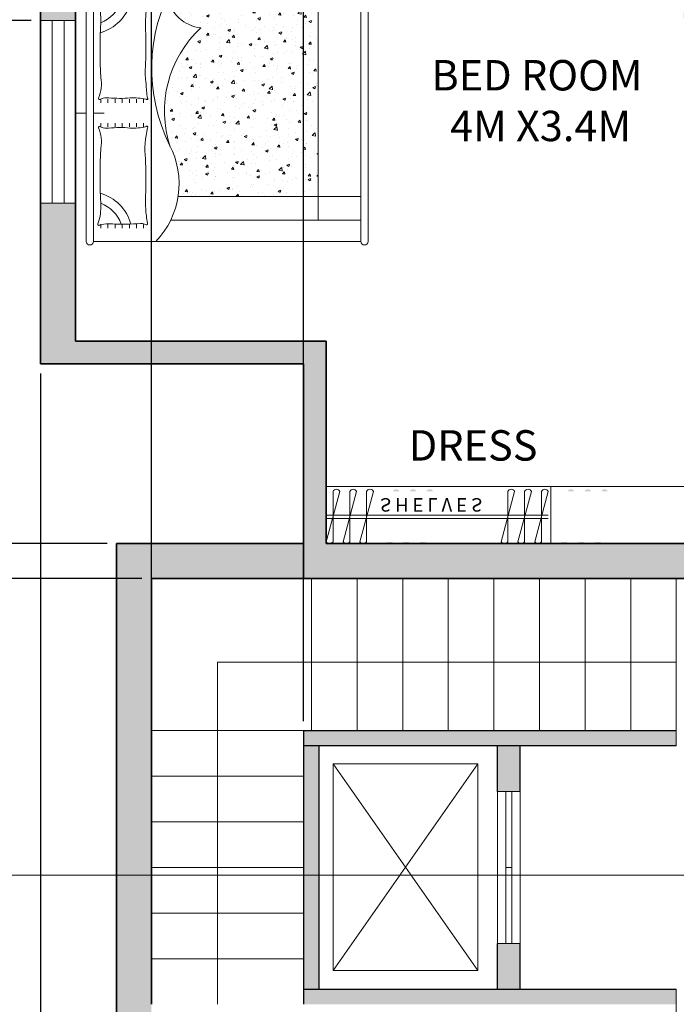
# Model space of a CAD drawing. Units: metres. Extents: x 2031 to 2061.8, y 1886.4 to 1909.8.
# Tile 5 of 10: x 2036.1 to 2040.4, y 1896.6 to 1903. Entities that reach past the tile are written whole.
import ezdxf

# ---------------------------------------------------------------- set-up
doc = ezdxf.new("R2010")
doc.units = ezdxf.units.M
for name, color, linetype, lineweight in [('A-ANNO-DIMS', 2, 'Continuous', 18), ('A-ANNO-SYMB', 7, 'Continuous', 18), ('A-AREA-IDEN', 7, 'Continuous', 18), ('A-FLOR-CASE', 8, 'Continuous', 18), ('A-FLOR-EVTR', 4, 'Continuous', 18), ('A-FLOR-STRS', 7, 'Continuous', 18), ('A-FLOR-STRS-PATH', 1, 'Continuous', 13), ('A-WALL-PATT', 252, 'Continuous', 13), ('furniture', 24, 'Continuous', 13), ('inner walls', 4, 'Continuous', 25), ('windows', 30, 'Continuous', 18)]:
    doc.layers.add(name, color=color, linetype=linetype, lineweight=lineweight)
doc.layers.add('outer walls', color=1, linetype='Continuous', lineweight=35, plot=False)
doc.styles.get("Standard").update_dxf_attribs({"font": 'arial.ttf'})
doc.dimstyles.get("Standard").update_dxf_attribs({"dimtxt": 0.18, "dimasz": 0.18, "dimexe": 0.18, "dimexo": 0.0625, "dimgap": 0.09, "dimtad": 0, "dimtih": 1, "dimtoh": 1, "dimdec": 4, "dimzin": 0, "dimdsep": 46, "dimtxsty": 'Standard', "dimcen": 0.09, "dimadec": 0, "dimazin": 0, "dimtfac": 1, "dimtdec": 4, "dimtofl": 0, "dimtmove": 0, "dimatfit": 3, "dimfxl": 1, "dimtolj": 1, "dimtzin": 0, "dimarcsym": 0})

# ---------------------------------------------------------------- blocks, each defined once
blk = doc.blocks.new('bed')
at = {"layer": 'furniture'}
h = blk.add_hatch(dxfattribs=at)
h.set_pattern_fill('AR-CONC', color=256, angle=-90.00000000000003, style=0)
h.set_pattern_definition([(320, (0, 2.380000000001032), (-0.6275213498259539, -7.172601826007534), [0.75, -8.25]), (265, (0, 2.380000000001032), (7.521921337000119, 1.387513336129997), [0.6, -6.599999999999999]), (10.45139999999999, (-0.0522933999999964, 1.782283200001032), (6.894395420609534, -5.785093817140218), [0.6374019000000001, -7.011421119999999]), (316.1842, (2, 2.380000000001032), (-1.655190143290184, -10.67241048625644), [1.125, -12.375]), (6.635599999999979, (1.862066929999997, 1.490632550001038), (9.741178709004412, -9.346627055487035), [0.956102879999999, -10.51712999999998]), (261.1842, (2, 2.380000000001032), (9.741186009253243, -9.346619451336275), [0.8999999999999989, -9.899999999999984]), (291, (1.5, 1.380000000001032), (-4.02618890665339, -5.969070521184614), [0.75, -8.25]), (236, (1.5, 1.380000000001032), (7.251500450468529, -2.433153319215819), [0.6, -6.599999999999999]), (341.4514, (1.164483939999996, 0.8825776700010266), (3.22530496709952, -8.402226285814901), [0.6374019000000001, -7.011421119999999]), (307.4999999999999, (0, 2.380000000001032), (3.328938538313114, -0.121598553172908), [0, -6.519999999999999, 0, -6.7, 0, -6.625]), (277.5, (0, 2.380000000001032), (3.944117118823601, -2.630695374421487), [0, -3.819999999999999, 0, -6.37, 0, -2.524999999999999]), (237.5, (0, 4.610000000001036), (-0.2255487173438, -5.33822436172409), [0, -2.5, 0, -7.799999999999999, 0, -10.35]), (227.5, (0, 5.610000000001036), (1.001049823323174, -5.831861693423862), [0, -3.25, 0, -5.179999999999999, 0, -7.349999999999999])])
h.paths.add_polyline_path([(30.01221964123038, -67.99999999999999), (30.01221964123036, -26.4972098666525, 0.2630430180581192), (23.90476957024844, -35.1500155485824, 0.2934236934375176), (-9.177957282599145, -26.46678060096597, -0.1566832162072435), (-23.39221964123496, -28.71851562074189), (-23.39221964123494, -67.99999999999999)])
for p, q in [((0, -3), (0, 0)), ((36.01221964123033, -3), (-36.01221964123033, -3)), ((-36.01221964123033, -5.000000000000028), (-36.01221964123027, -80)), ((36.01221964123033, -5.000000000000042), (-36.01221964123033, -5.000000000000028)), ((0, -8.000000000000043), (0, -5.000000000000042)), ((36.01221964123039, -79.99999999999999), (36.01221964123033, -5.000000000000042)), ((-31.23716250644156, -7.067621994530554), (-32.23716250644157, -7.067621994530554)), ((-3.810600647213163, -7.067621994530554), (-2.810600647213163, -7.067621994530554)), ((3.894900133777696, -7.067621994530526), (2.894900133777696, -7.067621994530526)), ((31.62837541028949, -7.067621994530526), (32.62837541028949, -7.067621994530526)), ((-31.23716250644156, -9.067621994530555), (-32.23716250644157, -9.067621994530555)), ((-3.810600647213163, -9.067621994530555), (-2.810600647213163, -9.067621994530555)), ((3.894900133777696, -9.067621994530526), (2.894900133777696, -9.067621994530526)), ((31.62837541028949, -9.067621994530526), (32.62837541028949, -9.067621994530526)), ((-31.23716250644156, -11.06762199453055), (-32.23716250644157, -11.06762199453055)), ((-31.23716250644156, -13.06762199453055), (-32.23716250644157, -13.06762199453055)), ((-3.810600647213163, -11.06762199453055), (-2.810600647213163, -11.06762199453055)), ((-3.810600647213163, -13.06762199453055), (-2.810600647213163, -13.06762199453055)), ((3.894900133777696, -11.06762199453052), (2.894900133777696, -11.06762199453052)), ((3.894900133777696, -13.06762199453052), (2.894900133777696, -13.06762199453052)), ((31.62837541028949, -11.06762199453052), (32.62837541028949, -11.06762199453052)), ((31.62837541028949, -13.06762199453052), (32.62837541028949, -13.06762199453052)), ((-31.23716250644156, -15.06762199453055), (-32.23716250644157, -15.06762199453055)), ((-3.810600647213163, -15.06762199453055), (-2.810600647213163, -15.06762199453055)), ((3.894900133777696, -15.06762199453052), (2.894900133777696, -15.06762199453052)), ((31.62837541028949, -15.06762199453052), (32.62837541028949, -15.06762199453052)), ((-31.23716250644156, -17.06762199453055), (-32.23716250644157, -17.06762199453055)), ((-31.23716250644156, -19.06762199453055), (-32.23716250644157, -19.06762199453055)), ((-3.810600647213163, -17.06762199453055), (-2.810600647213163, -17.06762199453055)), ((-3.810600647213163, -19.06762199453055), (-2.810600647213163, -19.06762199453055)), ((3.894900133777696, -17.06762199453052), (2.894900133777696, -17.06762199453052)), ((3.894900133777696, -19.06762199453052), (2.894900133777696, -19.06762199453052)), ((31.62837541028949, -17.06762199453052), (32.62837541028949, -17.06762199453052)), ((31.62837541028949, -19.06762199453052), (32.62837541028949, -19.06762199453052)), ((-36.01221964123027, -80), (36.01221964123039, -79.99999999999997)), ((-36.01221964123027, -82), (36.01221964123039, -82))]:
    blk.add_line(p, q, dxfattribs=at)
at = {"layer": 'furniture', "ltscale": 5}
blk.add_line((-30.0122196412303, -26.65900214866815), (-30.01221964123028, -80), dxfattribs=at)
at = {"layer": 'furniture', "ltscale": 7}
blk.add_line((30.01221964123039, -79.99999999999999), (30.01221964123036, -26.4972098666525), dxfattribs=at)
at = {"layer": 'furniture', "ltscale": 0.3}
for p, q in [((-23.39221964123493, -80.00000000000003), (-23.39221964123496, -28.71851562074188)), ((-30.01221964123028, -67.99999999999999), (30.01221964123039, -67.99999999999999))]:
    blk.add_line(p, q, dxfattribs=at)
at = {"layer": 'furniture'}
for centre, radius, start, end in [((-35.95310404783035, -4.000000000000014), 1.001745802777857, 93.38313670775338, 266.6168632922466), ((35.95310404783047, -4.000000000000014), 1.001745802777857, 273.3831367077534, 86.61686329224663), ((-31.09685452420217, -6.56812628935117), 0.3815901177143176, 35.89755946985184, 208.6271807330242), ((-44.4434251214767, -13.85312857714783), 14.82374463825802, 27.16285943351717, 28.62718073212637), ((-46.75951437957865, -9.65138206848897), 15.71579241958107, 357.4803608088326, 9.395608387614068), ((-34.45294545533051, -3.506108501804959), 9.853247350176973, 289.8695209624031, 338.9842964810487), ((-34.45294545533051, -3.506108501804959), 12.47479548168961, 286.0319050224358, 344.1205283884622), ((-26.34909713879518, 6.677823774407073), 13.75788850886336, 251.1782289026713, 273.3982224065857), ((-18.01528168092849, -163.5963416214672), 156.7209082093599, 87.00321809951629, 92.74968346925495), ((-8.031939823939297, 2.030581047412752), 9.294330538692307, 258.8960367609226, 294.7184225587751), ((0.254091396095987, -8.800915214962217), 4.494229367051207, 159.014640107615, 186.2730421081171), ((-4.029449448298862, -6.668977911985379), 0.2818061021667602, 335.7259061638442, 114.3030308467571), ((3.223958981487498, -9.94006998173215), 7.675076275868892, 155.7259061638442, 159.0146401085631), ((4.113748934860268, -6.668977911985379), 0.2818061021635516, 65.69696915417202, 204.2740938370052), ((-3.139659494904833, -9.940069981732137), 7.675076275868892, 20.98535989143595, 24.27409383615427), ((-0.1697919095242355, -8.800915214962217), 4.494229367051207, 353.7269578918828, 20.98535989238499), ((8.116239310533615, 2.030581047735168), 9.294330539002221, 245.2815774418415, 281.1039632384965), ((18.09958116748922, -163.5963416214399), 156.7209082093326, 87.2503165307418, 92.99678190048373), ((34.53724494190226, -3.506108501789682), 12.47479548168961, 195.8794716115377, 253.9680949775642), ((34.53724494190226, -3.506108501789682), 9.853247350176973, 201.0157035189505, 250.1304790375968), ((26.43339662535652, 6.677823774423444), 13.75788850886336, 266.6017775934111, 288.8217710973251), ((31.18115401076358, -6.568126289351184), 0.3815901177179044, 331.3728192669758, 144.1024405301472), ((46.84381386614001, -9.651382068520647), 15.71579241958353, 170.6043916115409, 182.5196391911672), ((44.52772460803806, -13.85312857714784), 14.82374463825802, 151.3728192678729, 152.8371405664821), ((54.88285648445511, -13.16191061182081), 85.98801403775587, 178.1208768196816, 183.3613129440673), ((-32.81622258778788, -12.43616332427339), 28.77528664700029, 354.3784002715227, 6.27304210895588), ((32.90052207435963, -12.43616332427341), 28.77528664700055, 173.7269578910441, 185.6215997284773), ((-54.79855699787332, -13.1619106118885), 85.98801403775471, 356.6386870559327, 1.87912318031836), ((-28.61556435462791, 31.03444768063454), 42.31456350822244, 266.4835611990511, 266.6487421238194), ((28.69986384117891, 31.03444768073385), 42.31456350831875, 273.3512578762066, 273.5164388009489), ((12.27920019974715, -16.10835590841725), 16.48064095036883, 177.0317121189266, 192.8677860199701), ((-12.19490071317551, -16.10835590841725), 16.48064095036894, 347.1322139800299, 2.968287881073314), ((-34.12771521855714, -18.41167218428833), 3.177308659740759, 342.7808628527732, 3.755021134780372), ((34.21201470513921, -18.41167218428845), 3.177308659740705, 176.2449788652196, 197.2191371472267), ((-31.05019458355673, -19.91479358257859), 0.2912925215689113, 147.6219291273817, 311.93432899363), ((-33.19532486499685, -18.55460390606353), 2.248727139855352, 327.6219291288709, 339.224552802207), ((-24.39731400277299, -58.0065508966982), 38.42172354635978, 93.51643880178425, 99.67664784205135), ((-24.51665474671893, -56.06449133928439), 36.47600066328987, 86.48356119821578, 93.51643880178425), ((-18.48842024981553, 70.49496359167773), 90.23180174042126, 267.5920770069633, 273.6328801943956), ((-10.30534078399284, -44.95285539311296), 25.51674577343078, 75.95197577712642, 95.54518109318596), ((12.50744191168894, -69.71437404891591), 48.3828132966499, 60.93454900685955, 116.3226601669859), ((-3.947726608991956, -19.99033763805275), 0.2654728058058112, 231.9004795059564, 52.89022406852256), ((4.032026095563765, -19.99033763805275), 0.2654728058058112, 127.1097759314774, 308.0995204940429), ((7.570216687580227, -34.67789736270967), 14.86666553287629, 87.39755039330738, 103.1191401867811), ((11.43897390287765, -34.80624327566366), 15.31635237680183, 84.69404282866213, 102.035481886755), ((18.57271973638731, 70.4949635916777), 90.23180174042125, 266.3671198056044, 272.4079229930367), ((24.6009542333012, -56.0644913392844), 36.47600066328987, 86.48356119821578, 93.51643880178425), ((24.48161348934542, -58.00655089669821), 38.42172354635978, 80.32335215794863, 86.48356119821578), ((31.13449407013883, -19.91479358255678), 0.2912925215689113, 228.06567100637, 32.37807087261824), ((33.27962435157895, -18.55460390604825), 2.248727139855352, 200.775447197793, 212.378070871129), ((-19.78970084288576, -5.469494448941333), 23.52647715105876, 226.4060518471351, 297.4441169484015), ((0.602167516954296, -56.56840710701565), 31.65057281321388, 42.58740832788977, 108.5033645785765), ((34.6132349005153, -36.22659364526982), 10.76244628919441, 101.1719081394, 174.2590453022261), ((-35.95310404783035, -81), 1.001745802777857, 93.38313670775338, 266.6168632922466), ((35.95310404783044, -81), 1.001745802777857, 273.3831367077534, 86.61686329224663)]:
    blk.add_arc(centre, radius, start, end, dxfattribs=at)
blk = doc.blocks.new('hangers')
at = {"layer": 'furniture'}
for p, q in [((1.8e-15, 16.5), (4.000000000000001, 1.5)), ((2.000000000000001, 16.5), (2.000000000000001, 1.5)), ((5.000000000000001, 16.5), (9.000000000000002, 1.5)), ((7.000000000000001, 16.5), (7.000000000000001, 1.5)), ((10, 16.5), (14, 1.5)), ((12, 16.5), (12, 1.5)), ((52, 16.5), (56, 1.5)), ((54, 16.5), (54, 1.5)), ((57, 16.5), (61, 1.5)), ((59, 16.5), (59, 1.5)), ((62, 16.5), (66, 1.5)), ((64, 16.5), (64, 1.5)), ((66, 9.5), (1.8e-15, 9.5)), ((1.8e-15, 8.5), (66, 8.5))]:
    blk.add_line(p, q, dxfattribs=at)
for centre, radius, start, end in [((1.000000000000001, 15.6218374153911), 1.33085293139661, 41.28839256573093, 138.711607434269), ((6.000000000000001, 15.6218374153911), 1.33085293139661, 41.28839256573093, 138.711607434269), ((11, 15.6218374153911), 1.33085293139661, 41.28839256573093, 138.711607434269), ((53, 15.6218374153911), 1.33085293139661, 41.28839256573107, 138.7116074342689), ((58, 15.6218374153911), 1.33085293139661, 41.28839256573107, 138.7116074342689), ((63, 15.6218374153911), 1.33085293139661, 41.28839256573107, 138.7116074342689), ((3.000000000000001, 1.915335972440686), 1.082822224561017, 202.5548696812492, 337.4451303187508), ((8.000000000000002, 1.915335972440686), 1.082822224561017, 202.5548696812492, 337.4451303187508), ((13, 1.915335972440686), 1.082822224561017, 202.5548696812492, 337.4451303187508), ((55, 1.915335972440686), 1.082822224561017, 202.5548696812491, 337.4451303187509), ((60, 1.915335972440686), 1.082822224561017, 202.5548696812491, 337.4451303187509), ((65, 1.915335972440686), 1.082822224561017, 202.5548696812491, 337.4451303187509)]:
    blk.add_arc(centre, radius, start, end, dxfattribs=at)
blk.add_point((0, 0), dxfattribs=at)
blk.add_text('S H E L V E S', height=4, dxfattribs=at).set_placement((15.9969173169515, 3.475366291579639))
blk = doc.blocks.new('WIN-1200')
for p, q in [((0.2299999999995634, 1.200000000000045), (-4.547e-13, 1.199999999999818)), ((0.0750000000007276, -2.274e-13), (0.0749999999995907, 1.200000000000045)), ((0.1550000000006548, -2.274e-13), (0.154999999999518, 1.200000000000045)), ((0.2300000000007003, 0), (6.821e-13, -2.274e-13))]:
    blk.add_line(p, q)
blk = doc.blocks.new('LIFT-CAR-PLAN')
for p, q in [((0.9511966047100486, -2.274e-13), (-2.274e-13, 1.357477288874861)), ((-2.274e-13, -2.274e-13), (0.9511966047100486, 1.357477288874861))]:
    blk.add_line(p, q)
blk.add_lwpolyline([(-2.274e-13, 1.357477288874861), (0.9511966047100486, 1.357477288874861), (0.9511966047100486, -2.274e-13), (-2.274e-13, -2.274e-13)], close=True)
blk = doc.blocks.new('*D44')
at = {"layer": 'A-ANNO-DIMS', "color": 0, "lineweight": -2, "transparency": 16777216}
for p, q in [((2036.232783, 1900.719895), (2036.232783, 1886.390195)), ((2056.453886, 1889.9931), (2056.453886, 1886.390195)), ((2036.412783, 1886.570195), (2045.94901662824, 1886.570195)), ((2056.273886, 1886.570195), (2046.73765237176, 1886.570195))]:
    blk.add_line(p, q, dxfattribs=at)
at = {"layer": 'A-ANNO-DIMS', "color": 0, "transparency": 16777216}
for points in [[(2036.412783, 1886.600195), (2036.412783, 1886.540195), (2036.232783, 1886.570195)], [(2056.273886, 1886.600195), (2056.273886, 1886.540195), (2056.453886, 1886.570195)]]:
    blk.add_solid(points, dxfattribs=at)
at = {"layer": 'Defpoints', "color": 0, "transparency": 16777216}
for p in [(2036.232783, 1900.782395), (2056.453886, 1890.0556), (2056.453886, 1886.570195)]:
    blk.add_point(p, dxfattribs=at)
at = {"layer": 'A-ANNO-DIMS', "color": 0, "transparency": 16777216, "insert": (2046.3433345, 1886.570195), "char_height": 0.18, "attachment_point": 5}
blk.add_mtext('\\A1;20.22', dxfattribs=at)
blk = doc.blocks.new('*D51')
at = {"layer": 'A-ANNO-DIMS', "color": 0, "lineweight": -2, "transparency": 16777216}
for p, q in [((2036.900694000001, 1899.371203000001), (2031.564780000002, 1899.371203000001)), ((2031.744780000002, 1899.191203000001), (2031.744780000002, 1897.653172529332)), ((2031.744780000002, 1895.751213000001), (2031.744780000002, 1897.289243470669)), ((2036.900694000001, 1895.571213000001), (2031.564780000002, 1895.571213000001))]:
    blk.add_line(p, q, dxfattribs=at)
at = {"layer": 'A-ANNO-DIMS', "color": 0, "transparency": 16777216}
for points in [[(2031.714780000002, 1899.191203000001), (2031.774780000002, 1899.191203000001), (2031.744780000002, 1899.371203000001)], [(2031.714780000002, 1895.751213000001), (2031.774780000002, 1895.751213000001), (2031.744780000002, 1895.571213000001)]]:
    blk.add_solid(points, dxfattribs=at)
at = {"layer": 'Defpoints', "color": 0, "transparency": 16777216}
for p in [(2031.744780000002, 1899.371203000001), (2036.963194000001, 1899.371203000001), (2036.963194000001, 1895.571213000001)]:
    blk.add_point(p, dxfattribs=at)
at = {"layer": 'A-ANNO-DIMS', "color": 0, "transparency": 16777216, "insert": (2031.744780000002, 1897.471207999999), "char_height": 0.18, "attachment_point": 5}
blk.add_mtext('\\A1;3.8', dxfattribs=at)
blk = doc.blocks.new('*D52')
at = {"layer": 'A-ANNO-DIMS', "color": 0, "lineweight": -2, "transparency": 16777216}
for p, q in [((2036.171386000001, 1903.039003000001), (2031.564780000002, 1903.039003000001)), ((2031.744780000002, 1902.859003000001), (2031.744780000002, 1901.502067529332)), ((2031.744780000002, 1899.781203000001), (2031.744780000002, 1901.138138470669)), ((2036.670694000001, 1899.601203000001), (2031.564780000002, 1899.601203000001))]:
    blk.add_line(p, q, dxfattribs=at)
at = {"layer": 'A-ANNO-DIMS', "color": 0, "transparency": 16777216}
for points in [[(2031.714780000002, 1902.859003000001), (2031.774780000002, 1902.859003000001), (2031.744780000002, 1903.039003000001)], [(2031.714780000002, 1899.781203000001), (2031.774780000002, 1899.781203000001), (2031.744780000002, 1899.601203000001)]]:
    blk.add_solid(points, dxfattribs=at)
at = {"layer": 'Defpoints', "color": 0, "transparency": 16777216}
for p in [(2031.744780000002, 1903.039003000001), (2036.233886000001, 1903.039003000001), (2036.733194000001, 1899.601203000001)]:
    blk.add_point(p, dxfattribs=at)
at = {"layer": 'A-ANNO-DIMS', "color": 0, "transparency": 16777216, "insert": (2031.744780000002, 1901.320102999999), "char_height": 0.18, "attachment_point": 5}
blk.add_mtext('\\A1;3.438', dxfattribs=at)
blk = doc.blocks.new('*D53')
at = {"layer": 'A-ANNO-DIMS', "color": 0, "lineweight": -2, "transparency": 16777216}
for p, q in [((2036.171386000001, 1904.659424000001), (2031.564780000002, 1904.659424000001)), ((2031.744780000002, 1904.479424000001), (2031.744780000002, 1904.031116637791)), ((2031.744780000002, 1903.219003000001), (2031.744780000002, 1903.667310362211)), ((2036.171386000001, 1903.039003000001), (2031.564780000002, 1903.039003000001))]:
    blk.add_line(p, q, dxfattribs=at)
at = {"layer": 'A-ANNO-DIMS', "color": 0, "transparency": 16777216}
for points in [[(2031.714780000002, 1904.479424000001), (2031.774780000002, 1904.479424000001), (2031.744780000002, 1904.659424000001)], [(2031.714780000002, 1903.219003000001), (2031.774780000002, 1903.219003000001), (2031.744780000002, 1903.039003000001)]]:
    blk.add_solid(points, dxfattribs=at)
at = {"layer": 'Defpoints', "color": 0, "transparency": 16777216}
for p in [(2031.744780000002, 1904.659424000001), (2036.233886000001, 1904.659424000001), (2036.233886000001, 1903.039003000001)]:
    blk.add_point(p, dxfattribs=at)
at = {"layer": 'A-ANNO-DIMS', "color": 0, "transparency": 16777216, "insert": (2031.744780000002, 1903.8492135), "char_height": 0.18, "attachment_point": 5}
blk.add_mtext('\\A1;1.62', dxfattribs=at)
blk = doc.blocks.new('*D59')
at = {"layer": 'A-ANNO-DIMS', "color": 0, "lineweight": -2, "transparency": 16777216}
for p, q in [((2036.963194, 1898.433713), (2036.963194, 1909.84065)), ((2037.963194, 1898.433713), (2037.963194, 1909.84065)), ((2037.143194, 1909.66065), (2037.340042567531, 1909.66065)), ((2037.783194, 1909.66065), (2037.586345432469, 1909.66065))]:
    blk.add_line(p, q, dxfattribs=at)
at = {"layer": 'A-ANNO-DIMS', "color": 0, "transparency": 16777216}
for points in [[(2037.143194, 1909.69065), (2037.143194, 1909.63065), (2036.963194, 1909.66065)], [(2037.783194, 1909.69065), (2037.783194, 1909.63065), (2037.963194, 1909.66065)]]:
    blk.add_solid(points, dxfattribs=at)
at = {"layer": 'Defpoints', "color": 0, "transparency": 16777216}
for p in [(2037.963194, 1909.66065), (2036.963194, 1898.371213), (2037.963194, 1898.371213)]:
    blk.add_point(p, dxfattribs=at)
at = {"layer": 'A-ANNO-DIMS', "color": 0, "transparency": 16777216, "insert": (2037.463194, 1909.66065), "char_height": 0.18, "attachment_point": 5}
blk.add_mtext('\\A1;1', dxfattribs=at)

msp = doc.modelspace()

# ---------------------------------------------------------------- hatches: boundary and pattern name
at = {"layer": 'A-WALL-PATT'}
h = msp.add_hatch(color=256, dxfattribs=at)
h.dxf.hatch_style = 1
h.paths.add_polyline_path([(2044.843886051581, 1905.431202972395), (2043.662726773602, 1905.431202972395), (2043.662726773602, 1905.201202972395), (2044.613886051581, 1905.201202972395), (2044.613886051581, 1903.201202972395), (2044.10203621828, 1903.201202972395), (2044.10203621828, 1903.051247813867), (2044.613886051581, 1903.051202972395), (2044.613784550147, 1901.892599367488), (2044.843481671829, 1901.892599367488)])
h.paths.add_polyline_path([(2044.843886051581, 1907.081202972395), (2044.693886051581, 1907.081202972395), (2044.693886051581, 1905.431202972395), (2044.843886051581, 1905.431202972395)])
h.paths.add_polyline_path([(2042.662726773602, 1905.431202972395), (2041.608725591668, 1905.431202972395), (2041.608725591668, 1905.201202972395), (2042.113886051581, 1905.201202972395), (2042.113886051581, 1903.201202972395), (2042.11388605158, 1903.200960518025), (2041.878665859902, 1903.200960518025, -0.0160568248018428), (2041.87111792116, 1903.201202972395), (2040.613886051581, 1903.201202972395), (2040.463886051581, 1903.201202972395), (2040.46388605158, 1903.051202972395), (2042.263886051581, 1903.051202972395), (2042.263886051581, 1905.201202972395), (2042.662726773602, 1905.201202972395)])
h.paths.add_polyline_path([(2040.804457664849, 1903.878793012381), (2041.776183449296, 1903.878793012381), (2041.776183449296, 1904.438513339803), (2040.804457664849, 1904.438513339803)], flags=25)
h.paths.add_polyline_path([(2042.05521314868, 1900.945611707966), (2043.754121743495, 1900.945611707966), (2043.754121743495, 1901.691905477861), (2042.05521314868, 1901.691905477861)], flags=9)
h.paths.add_polyline_path([(2038.540886554753, 1905.248744193212), (2040.159440442883, 1905.248744193212), (2040.159440442883, 1905.995037963107), (2038.540886554753, 1905.995037963107)], flags=9)
h.paths.add_polyline_path([(2038.693906317999, 1902.140700941841), (2040.392814912815, 1902.140700941841), (2040.392814912815, 1902.886994711737), (2038.693906317999, 1902.886994711737)], flags=9)
h.paths.add_polyline_path([(2042.359230799286, 1903.821641126969), (2043.685560949354, 1903.821641126969), (2043.685560949354, 1904.567934896864), (2042.359230799286, 1904.567934896864)], flags=9)
h = msp.add_hatch(color=256, dxfattribs=at)
h.dxf.hatch_style = 1
h.paths.add_polyline_path([(2037.96388605158, 1906.2440838694), (2037.96388605158, 1906.3940838694), (2037.81388605158, 1906.3940838694), (2037.81388605158, 1904.659423662096), (2036.233886051581, 1904.659423662097), (2036.233425041249, 1903.039002867159), (2036.463447491671, 1903.039002867159), (2036.463886051581, 1904.429423662097), (2039.563886051581, 1904.429423662097), (2039.563886051581, 1904.659423662097), (2037.96388605158, 1904.659423662097)])
h = msp.add_hatch(color=256, dxfattribs=at)
h.dxf.hatch_style = 1
h.paths.add_polyline_path([(2044.843367395183, 1900.892599367488), (2044.61369694345, 1900.892599367488), (2044.61356365894, 1899.371202985826), (2044.843193535108, 1899.371202985826)])
h.paths.add_polyline_path([(2041.161147521447, 1899.371202985826), (2041.161147521447, 1899.601202985826), (2040.68737920617, 1899.601202985827), (2040.68737920617, 1899.976202985826), (2040.687485090836, 1900.265858024963), (2040.53737920617, 1900.265912896825), (2040.53737920617, 1899.601202985826), (2038.113193535108, 1899.601202985827), (2038.112783035539, 1900.932395301215), (2036.462783035539, 1900.932395301215), (2036.463068993382, 1901.839002867159), (2036.233083640793, 1901.839002867159), (2036.232783035539, 1900.782395301215), (2037.962783035539, 1900.782395301215), (2037.963193535108, 1899.371202985826)])
h = msp.add_hatch(color=256, dxfattribs=at)
h.dxf.hatch_style = 1
h.paths.add_polyline_path([(2043.413579428145, 1899.371202985826), (2043.413579428145, 1899.551202985826), (2043.414968643082, 1899.601202985826), (2042.361147521447, 1899.601202985826), (2042.361147521447, 1899.371202985826)])
edge = h.paths.add_edge_path()
edge.add_line((2038.506381150364, 1899.788201292628), (2039.966159003426, 1899.788201292628))
edge = h.paths.add_edge_path()
edge.add_line((2039.966159003426, 1899.766083446369), (2038.506381150364, 1899.766083446369))
edge = h.paths.add_edge_path()
edge.add_arc((2038.528498996622, 1899.630681587596), 0.0294356005293348, 221.2883925659197, 318.7116074340803)
edge = h.paths.add_edge_path()
edge.add_arc((2038.572734689139, 1899.933839879253), 0.0239496954881524, 22.5548696809955, 157.4451303190045)
edge = h.paths.add_edge_path()
edge.add_line((2038.506381150364, 1899.61125852256), (2038.594852535398, 1899.943026216438))
edge = h.paths.add_edge_path(flags=17)
edge.add_line((2038.550616842881, 1899.61125852256), (2038.550616842881, 1899.943026216438))
edge = h.paths.add_edge_path()
edge.add_arc((2038.639088227915, 1899.630681587596), 0.0294356005293348, 221.2883925659197, 318.7116074340803)
edge = h.paths.add_edge_path()
edge.add_arc((2038.683323920432, 1899.933839879253), 0.0239496954881524, 22.5548696809955, 157.4451303190045)
edge = h.paths.add_edge_path()
edge.add_line((2038.616970381656, 1899.61125852256), (2038.70544176669, 1899.943026216438))
edge = h.paths.add_edge_path(flags=17)
edge.add_line((2038.661206074174, 1899.61125852256), (2038.661206074174, 1899.943026216438))
edge = h.paths.add_edge_path()
edge.add_arc((2038.749677459207, 1899.630681587596), 0.0294356005293348, 221.2883925659197, 318.7116074340803)
edge = h.paths.add_edge_path()
edge.add_arc((2038.793913151724, 1899.933839879253), 0.0239496954881524, 22.5548696809955, 157.4451303190045)
edge = h.paths.add_edge_path()
edge.add_line((2038.727559612949, 1899.61125852256), (2038.816030997983, 1899.943026216438))
edge = h.paths.add_edge_path(flags=17)
edge.add_line((2038.771795305466, 1899.61125852256), (2038.771795305466, 1899.943026216438))
edge = h.paths.add_edge_path()
edge.add_arc((2039.678627002065, 1899.630681587596), 0.0294356005293348, 221.2883925659197, 318.7116074340803)
edge = h.paths.add_edge_path()
edge.add_arc((2039.722862694583, 1899.933839879253), 0.0239496954881524, 22.5548696809955, 157.4451303190045)
edge = h.paths.add_edge_path()
edge.add_line((2039.656509155807, 1899.61125852256), (2039.744980540841, 1899.943026216438))
edge = h.paths.add_edge_path(flags=17)
edge.add_line((2039.700744848324, 1899.61125852256), (2039.700744848324, 1899.943026216438))
edge = h.paths.add_edge_path()
edge.add_arc((2039.789216233358, 1899.630681587596), 0.0294356005293348, 221.2883925659197, 318.7116074340803)
edge = h.paths.add_edge_path()
edge.add_arc((2039.833451925875, 1899.933839879253), 0.0239496954881524, 22.5548696809955, 157.4451303190045)
edge = h.paths.add_edge_path()
edge.add_line((2039.7670983871, 1899.61125852256), (2039.855569772134, 1899.943026216438))
edge = h.paths.add_edge_path(flags=17)
edge.add_line((2039.811334079616, 1899.61125852256), (2039.811334079616, 1899.943026216438))
edge = h.paths.add_edge_path()
edge.add_arc((2039.899805464651, 1899.630681587596), 0.0294356005293348, 221.2883925659197, 318.7116074340803)
edge = h.paths.add_edge_path()
edge.add_arc((2039.944041157168, 1899.933839879253), 0.0239496954881524, 22.5548696809955, 157.4451303190045)
edge = h.paths.add_edge_path()
edge.add_line((2039.877687618392, 1899.61125852256), (2039.966159003426, 1899.943026216438))
edge = h.paths.add_edge_path(flags=17)
edge.add_line((2039.921923310909, 1899.61125852256), (2039.921923310909, 1899.943026216438))
h.paths.add_polyline_path([(2038.837326301555, 1899.786483056072), (2039.659277368514, 1899.786483056072), (2039.659277368514, 1899.923716295886), (2038.837326301555, 1899.923716295886)], flags=9)
h = msp.add_hatch(color=256, dxfattribs=at)
h.dxf.hatch_style = 1
h.paths.add_polyline_path([(2036.963193532321, 1899.371202985826), (2037.963193535108, 1899.371202985826), (2037.96312663076, 1899.601202985826), (2036.733193532321, 1899.601202985826), (2036.733193532322, 1895.341212564149), (2040.415704939613, 1895.341212564148), (2040.415704939613, 1895.571212564149), (2038.015704939613, 1895.571212564149), (2036.963193532321, 1895.571212564149), (2036.963193532321, 1896.571212564148), (2036.963193532321, 1898.371212564148)])
h.paths.add_polyline_path([(2038.063193532321, 1898.271212564148), (2040.415704939613, 1898.271212564148), (2040.415704939613, 1898.371212564148), (2037.963193532322, 1898.371212564148), (2037.963193532322, 1896.571212564149), (2040.415704939613, 1896.571212564149), (2040.415704939613, 1896.671212564148), (2038.063193532321, 1896.671212564148)], flags=17)
h = msp.add_hatch(color=256, dxfattribs=at)
h.dxf.hatch_style = 1
h.paths.add_polyline_path([(2039.389449235967, 1896.971212564148), (2039.239449235967, 1896.971212564148), (2039.239449235967, 1896.671212564148), (2039.389449235967, 1896.671212564148)])
h.paths.add_polyline_path([(2039.389449235967, 1898.271212564148), (2039.239449235967, 1898.271212564148), (2039.239449235967, 1897.971212564149), (2039.389449235967, 1897.971212564149)])

# ---------------------------------------------------------------- linework, layer by layer
at = {"layer": 'A-ANNO-SYMB'}
msp.add_line((2033.125780009863, 1897.420015762724), (2060.053374346622, 1897.420015762724), dxfattribs=at)
at = {"layer": 'A-FLOR-CASE', "ltscale": 0.3}
msp.add_line((2038.113193535108, 1899.976202985826), (2040.53737920617, 1899.976202985826), dxfattribs=at)
at = {"layer": 'A-FLOR-CASE'}
msp.add_line((2039.591011168068, 1899.601202985827), (2039.591011168068, 1899.976202985826), dxfattribs=at)
at = {"layer": 'A-FLOR-EVTR'}
for p, q in [((2039.389449235967, 1897.971212564149), (2039.239449235967, 1897.971212564149)), ((2039.389449235967, 1896.971212564148), (2039.239449235967, 1896.971212564148))]:
    msp.add_line(p, q, dxfattribs=at)
for points in [[(2039.239449235967, 1896.971212564148), (2039.239449235967, 1897.971212564149)], [(2039.294449235967, 1896.971212564148), (2039.294449235967, 1897.971212564149)], [(2039.334449235967, 1896.971212564148), (2039.334449235967, 1897.971212564149)], [(2039.389449235967, 1896.971212564148), (2039.389449235967, 1897.971212564149)], [(2039.334449235967, 1897.471212564148), (2039.294449235967, 1897.471212564148)]]:
    msp.add_lwpolyline(points, dxfattribs=at)
at = {"layer": 'A-FLOR-STRS'}
for p, q in [((2038.015704939613, 1899.371212564148), (2038.015704939613, 1898.371212564148)), ((2038.315704939613, 1899.371212564148), (2038.315704939613, 1898.371212564148)), ((2038.615704939613, 1899.371212564148), (2038.615704939613, 1898.371212564148)), ((2038.915704939613, 1899.371212564148), (2038.915704939613, 1898.371212564148)), ((2039.215704939613, 1899.371212564148), (2039.215704939613, 1898.371212564148)), ((2039.515704939613, 1899.371212564148), (2039.515704939613, 1898.371212564148)), ((2039.815704939613, 1899.371212564148), (2039.815704939613, 1898.371212564148)), ((2040.115704939613, 1899.371212564148), (2040.115704939613, 1898.371212564148)), ((2040.415704939613, 1899.371212564148), (2040.415704939613, 1898.271212564148)), ((2037.963193532322, 1898.371212564148), (2036.963193532321, 1898.371212564148)), ((2037.963193532322, 1898.071212564148), (2036.963193532321, 1898.071212564148)), ((2037.963193532322, 1897.771212564148), (2036.963193532321, 1897.771212564149)), ((2037.963193532322, 1897.471212564148), (2036.963193532321, 1897.471212564148)), ((2037.963193532322, 1897.171212564148), (2036.963193532321, 1897.171212564149)), ((2037.963193532322, 1896.871212564149), (2036.963193532321, 1896.871212564149)), ((2040.415704939613, 1896.671212564148), (2040.415704939613, 1895.341212564148))]:
    msp.add_line(p, q, dxfattribs=at)
at = {"layer": 'A-FLOR-STRS-PATH'}
for p, q in [((2040.415704939613, 1898.821212564148), (2037.398133785105, 1898.821212564148)), ((2037.398133785105, 1898.821212564148), (2037.398133785105, 1896.571212564148))]:
    msp.add_line(p, q, dxfattribs=at)
at = {"layer": 'inner walls'}
for p, q in [((2037.963193532322, 1898.371212564148), (2037.963193532322, 1896.571212564149)), ((2038.063193532321, 1898.271212564148), (2038.063193532321, 1896.671212564148)), ((2039.239449235967, 1897.971212564149), (2039.239449235967, 1898.271212564148)), ((2039.389449235967, 1897.971212564149), (2039.389449235967, 1898.271212564148)), ((2039.239449235967, 1896.671212564148), (2039.239449235967, 1896.971212564148)), ((2039.389449235967, 1896.671212564148), (2039.389449235967, 1896.971212564148))]:
    msp.add_line(p, q, dxfattribs=at)
for points in [[(2037.963193532322, 1898.371212564148), (2040.415704939613, 1898.371212564148)], [(2040.415704939613, 1898.271212564148), (2037.963193532322, 1898.271212564148)], [(2037.963193532322, 1896.671212564148), (2040.415704939613, 1896.671212564148)]]:
    msp.add_lwpolyline(points, dxfattribs=at)
at = {"layer": 'outer walls'}
for p, q in [((2036.233886051581, 1904.659423662097), (2036.232783035539, 1900.782395301215)), ((2036.463886051581, 1904.429423662097), (2036.462783035539, 1900.932395301215)), ((2036.462783035539, 1900.932395301215), (2038.112783035539, 1900.932395301215)), ((2038.112783035539, 1900.932395301215), (2038.113193535108, 1899.601202985827)), ((2036.232783035539, 1900.782395301215), (2037.962783035539, 1900.782395301215)), ((2037.962783035539, 1900.782395301215), (2037.963193535108, 1899.371202985826)), ((2037.963193535108, 1899.601202985826), (2036.733193532321, 1899.601202985826)), ((2036.733193532321, 1899.601202985826), (2036.733193532322, 1895.341212564149)), ((2038.113193535108, 1899.601202985827), (2040.537242123281, 1899.601202985826)), ((2037.963193535108, 1899.371202985826), (2036.963193532321, 1899.371202985826)), ((2036.963193532321, 1899.371202985826), (2036.963193532321, 1898.371212564148)), ((2037.963193535108, 1899.371202985826), (2043.414968643082, 1899.371202985826)), ((2036.963193532321, 1898.371212564148), (2036.963193532321, 1896.571212564148))]:
    msp.add_line(p, q, dxfattribs=at)

# ---------------------------------------------------------------- block references
at = {"layer": 'A-FLOR-CASE', "xscale": -0.022117846258523, "yscale": 0.022117846258523, "zscale": 0.022117846258523, "rotation": 180}
msp.add_blockref('hangers', (2038.113077933816, 1899.976081702973), dxfattribs=at)
at = {"layer": 'A-FLOR-EVTR'}
msp.add_blockref('LIFT-CAR-PLAN', (2038.158934321573, 1896.793865092853), dxfattribs=at)
at = {"layer": 'furniture', "xscale": 0.023464496412097, "yscale": 0.023464496412097, "zscale": 0.023464496412097, "rotation": 90.00000000000003}
msp.add_blockref('bed', (2036.463886051581, 1902.430910089979), dxfattribs=at)
at = {"layer": 'windows'}
msp.add_blockref('WIN-1200', (2036.233886051581, 1901.839002867159), dxfattribs=at)

# ---------------------------------------------------------------- texts
at = {"layer": 'A-AREA-IDEN', "char_height": 0.2, "attachment_point": 7}
for s, insert in [(' BED ROOM\\P   4M X3.4M', (2038.743906317999, 1902.246362606234)), ('   DRESS', (2038.471988028262, 1900.14591271352))]:
    msp.add_mtext_dynamic_manual_height_columns(s, width=2.302330104705106, gutter_width=12.5, heights=[0], dxfattribs=dict(at, insert=insert))

# ---------------------------------------------------------------- dimensions: what is measured, and where the dimension line sits
at = {"layer": 'A-ANNO-DIMS'}
for base, p1, p2, override, picture, middle in [((2037.963194, 1909.66065), (2036.963194, 1898.371213), (2037.963194, 1898.371213), {"dimdec": 0, "dimlfac": 1, "dimrnd": 0, "dimzin": 0, "dimdsep": 46, "dimlunit": 2}, '*D59', (2037.463194, 1909.66065)), ((2056.453886, 1886.570195), (2036.232783, 1900.782395), (2056.453886, 1890.0556), {"dimdec": 2, "dimlfac": 1, "dimrnd": 0, "dimzin": 0, "dimdsep": 46, "dimlunit": 2}, '*D44', (2046.3433345, 1886.570195))]:
    dim = msp.add_linear_dim(base=base, p1=p1, p2=p2, dimstyle='Standard', override=override, dxfattribs=at)
    dim.commit()
    dim.dimension.update_dxf_attribs({"geometry": picture, "text_midpoint": middle})
for base, p1, p2, override, picture, middle in [((2031.744780000002, 1904.659424000001), (2036.233886, 1903.039003), (2036.233886, 1904.659424), {"dimdec": 2, "dimlfac": 1, "dimrnd": 0, "dimzin": 0, "dimdsep": 46, "dimlunit": 2}, '*D53', (2031.744780000002, 1903.8492135)), ((2031.744780000002, 1903.039003000001), (2036.733194, 1899.601203), (2036.233886, 1903.039003), {"dimdec": 3, "dimlfac": 1, "dimrnd": 0, "dimzin": 0, "dimdsep": 46, "dimlunit": 2}, '*D52', (2031.744780000002, 1901.320102999999)), ((2031.744780000002, 1899.371203000001), (2036.963194, 1895.571213), (2036.963194, 1899.371203), {"dimdec": 1, "dimlfac": 1, "dimrnd": 0, "dimzin": 0, "dimdsep": 46, "dimlunit": 2}, '*D51', (2031.744780000002, 1897.471207999999))]:
    dim = msp.add_linear_dim(base=base, p1=p1, p2=p2, angle=90, dimstyle='Standard', override=override, dxfattribs=at)
    dim.commit()
    dim.dimension.update_dxf_attribs({"geometry": picture, "text_midpoint": middle})

doc.saveas('drawing.dxf')
